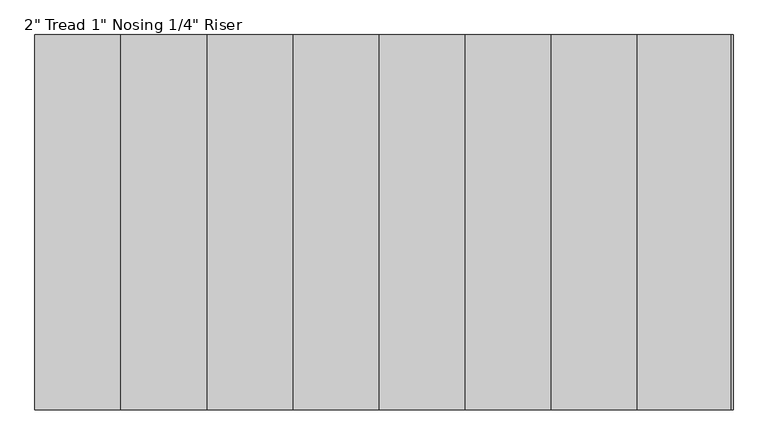
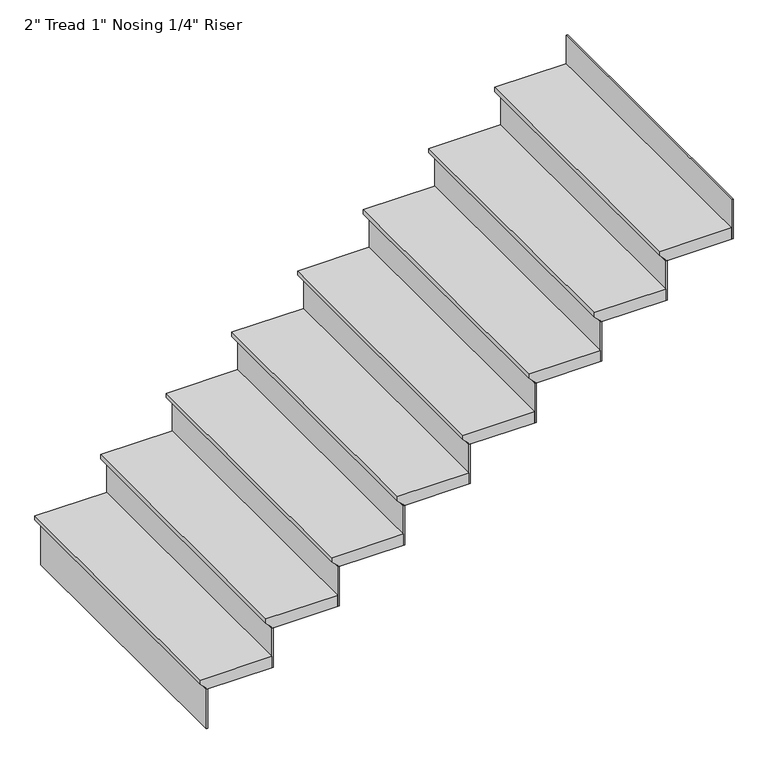
"""IFC4 building model written with IfcOpenShell, lengths in millimetres: stair flight geometry."""

from ifc_helpers import new_model, si_unit, frame, origin, place, context, project, spatial, polyline, outline, extrude, source, transform, mapped, element, save


def stair_flight_e2acd8df(model_context):
    return source(origin(), model_context, "Body", "SweptSolid", [
        extrude(outline(polyline([(4978.4, -7818.6707895), (4978.4, -8123.4707895), (4959.35, -8123.4707895), (4933.95, -8098.0707895), (4927.6, -8098.0707895), (4927.6, -7818.6707895), (4978.4, -7818.6707895)])), frame((0.0, 6461.9144188, 0.0), z_axis=(0.0, 1.0, 0.0), x_axis=(0.0, 0.0, 1.0)), (0.0, 0.0, 1.0), 1219.2),
        extrude(outline(polyline([(-8091.7207895, 6461.9144188), (-8098.0707895, 6461.9144188), (-8098.0707895, 7681.1144188), (-8091.7207895, 7681.1144188), (-8091.7207895, 6461.9144188)])), frame((0.0, 0.0, 4749.8), z_axis=(0.0, 0.0, 1.0), x_axis=(1.0, 0.0, 0.0)), (0.0, 0.0, 1.0), 177.8),
        extrude(outline(polyline([(-7812.3207895, 6461.9144188), (-7818.6707895, 6461.9144188), (-7818.6707895, 7681.1144188), (-7812.3207895, 7681.1144188), (-7812.3207895, 6461.9144188)])), frame((0.0, 0.0, 4927.6), z_axis=(0.0, 0.0, 1.0), x_axis=(1.0, 0.0, 0.0)), (0.0, 0.0, 1.0), 177.8),
        extrude(outline(polyline([(5156.2, -7539.2707895), (5156.2, -7844.0707895), (5137.15, -7844.0707895), (5111.75, -7818.6707895), (5105.4, -7818.6707895), (5105.4, -7539.2707895), (5156.2, -7539.2707895)])), frame((0.0, 6461.9144188, 0.0), z_axis=(0.0, 1.0, 0.0), x_axis=(0.0, 0.0, 1.0)), (0.0, 0.0, 1.0), 1219.2),
        extrude(outline(polyline([(-7532.9207895, 6461.9144188), (-7539.2707895, 6461.9144188), (-7539.2707895, 7681.1144188), (-7532.9207895, 7681.1144188), (-7532.9207895, 6461.9144188)])), frame((0.0, 0.0, 5105.4), z_axis=(0.0, 0.0, 1.0), x_axis=(1.0, 0.0, 0.0)), (0.0, 0.0, 1.0), 177.8),
        extrude(outline(polyline([(5334.0, -7259.8707895), (5334.0, -7564.6707895), (5314.95, -7564.6707895), (5289.55, -7539.2707895), (5283.2, -7539.2707895), (5283.2, -7259.8707895), (5334.0, -7259.8707895)])), frame((0.0, 6461.9144188, 0.0), z_axis=(0.0, 1.0, 0.0), x_axis=(0.0, 0.0, 1.0)), (0.0, 0.0, 1.0), 1219.2),
        extrude(outline(polyline([(-7253.5207895, 6461.9144188), (-7259.8707895, 6461.9144188), (-7259.8707895, 7681.1144188), (-7253.5207895, 7681.1144188), (-7253.5207895, 6461.9144188)])), frame((0.0, 0.0, 5283.2), z_axis=(0.0, 0.0, 1.0), x_axis=(1.0, 0.0, 0.0)), (0.0, 0.0, 1.0), 177.8),
        extrude(outline(polyline([(5511.8, -6980.4707895), (5511.8, -7285.2707895), (5492.75, -7285.2707895), (5467.35, -7259.8707895), (5461.0, -7259.8707895), (5461.0, -6980.4707895), (5511.8, -6980.4707895)])), frame((0.0, 6461.9144188, 0.0), z_axis=(0.0, 1.0, 0.0), x_axis=(0.0, 0.0, 1.0)), (0.0, 0.0, 1.0), 1219.2),
        extrude(outline(polyline([(-6974.1207895, 6461.9144188), (-6980.4707895, 6461.9144188), (-6980.4707895, 7681.1144188), (-6974.1207895, 7681.1144188), (-6974.1207895, 6461.9144188)])), frame((0.0, 0.0, 5461.0), z_axis=(0.0, 0.0, 1.0), x_axis=(1.0, 0.0, 0.0)), (0.0, 0.0, 1.0), 177.8),
        extrude(outline(polyline([(5689.6, -6701.0707895), (5689.6, -7005.8707895), (5670.55, -7005.8707895), (5645.15, -6980.4707895), (5638.8, -6980.4707895), (5638.8, -6701.0707895), (5689.6, -6701.0707895)])), frame((0.0, 6461.9144188, 0.0), z_axis=(0.0, 1.0, 0.0), x_axis=(0.0, 0.0, 1.0)), (0.0, 0.0, 1.0), 1219.2),
        extrude(outline(polyline([(-6694.7207895, 6461.9144188), (-6701.0707895, 6461.9144188), (-6701.0707895, 7681.1144188), (-6694.7207895, 7681.1144188), (-6694.7207895, 6461.9144188)])), frame((0.0, 0.0, 5638.8), z_axis=(0.0, 0.0, 1.0), x_axis=(1.0, 0.0, 0.0)), (0.0, 0.0, 1.0), 177.8),
        extrude(outline(polyline([(5867.4, -6421.6707895), (5867.4, -6726.4707895), (5848.35, -6726.4707895), (5822.95, -6701.0707895), (5816.6, -6701.0707895), (5816.6, -6421.6707895), (5867.4, -6421.6707895)])), frame((0.0, 6461.9144188, 0.0), z_axis=(0.0, 1.0, 0.0), x_axis=(0.0, 0.0, 1.0)), (0.0, 0.0, 1.0), 1219.2),
        extrude(outline(polyline([(-6415.3207895, 6461.9144188), (-6421.6707895, 6461.9144188), (-6421.6707895, 7681.1144188), (-6415.3207895, 7681.1144188), (-6415.3207895, 6461.9144188)])), frame((0.0, 0.0, 5816.6), z_axis=(0.0, 0.0, 1.0), x_axis=(1.0, 0.0, 0.0)), (0.0, 0.0, 1.0), 177.8),
        extrude(outline(polyline([(6045.2, -6142.2707895), (6045.2, -6447.0707895), (6026.15, -6447.0707895), (6000.75, -6421.6707895), (5994.4, -6421.6707895), (5994.4, -6142.2707895), (6045.2, -6142.2707895)])), frame((0.0, 6461.9144188, 0.0), z_axis=(0.0, 1.0, 0.0), x_axis=(0.0, 0.0, 1.0)), (0.0, 0.0, 1.0), 1219.2),
        extrude(outline(polyline([(-6135.9207895, 6461.9144188), (-6142.2707895, 6461.9144188), (-6142.2707895, 7681.1144188), (-6135.9207895, 7681.1144188), (-6135.9207895, 6461.9144188)])), frame((0.0, 0.0, 5994.4), z_axis=(0.0, 0.0, 1.0), x_axis=(1.0, 0.0, 0.0)), (0.0, 0.0, 1.0), 177.8),
        extrude(outline(polyline([(-5856.5207895, 6461.9144188), (-5862.8707895, 6461.9144188), (-5862.8707895, 7681.1144188), (-5856.5207895, 7681.1144188), (-5856.5207895, 6461.9144188)])), frame((0.0, 0.0, 6172.2), z_axis=(0.0, 0.0, 1.0), x_axis=(1.0, 0.0, 0.0)), (0.0, 0.0, 1.0), 177.8),
        extrude(outline(polyline([(6223.0, -5862.8707895), (6223.0, -6167.6707895), (6203.95, -6167.6707895), (6178.55, -6142.2707895), (6172.2, -6142.2707895), (6172.2, -5862.8707895), (6223.0, -5862.8707895)])), frame((0.0, 6461.9144188, 0.0), z_axis=(0.0, 1.0, 0.0), x_axis=(0.0, 0.0, 1.0)), (0.0, 0.0, 1.0), 1219.2),
    ])


if __name__ == "__main__":
    model = new_model("IFC4")
    model_context = context("Model", 3, world=origin())
    ifc_project = project(units=[si_unit("LENGTHUNIT", "METRE", prefix="MILLI")], contexts=[model_context])
    site = spatial("IfcSite", under=ifc_project)
    building = spatial("IfcBuilding", under=site)
    placement = place(None, origin())
    stair_flight_shape = stair_flight_e2acd8df(model_context)
    element("IfcStairFlight", 1, ObjectType="2\" Tread 1\" Nosing 1/4\" Riser", at=placement, inside=building, context=model_context, shape_type="MappedRepresentation", body=[
        mapped(stair_flight_shape, transform((0.0, 0.0, 0.0), x_axis=(1.0, 0.0, 0.0), y_axis=(0.0, 1.0, 0.0), z_axis=(0.0, 0.0, 1.0))),
    ])
    save(model, "model.ifc")
